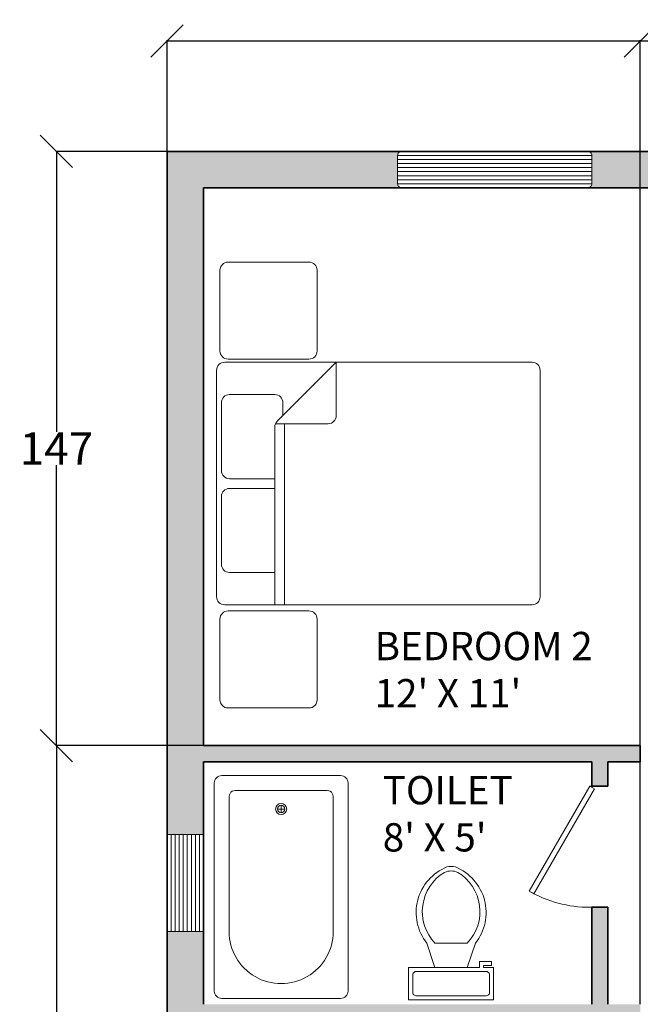
# Model space of a CAD drawing. Units: inches. Extents: x -8 to 447, y -560 to 47.
# Tile 3 of 5: x -8 to 146, y -196 to 47. Entities that reach past the tile are written whole.
import ezdxf

# ---------------------------------------------------------------- set-up
doc = ezdxf.new("R2010")
doc.units = ezdxf.units.IN
doc.header["$MEASUREMENT"] = 0
for name, color, linetype, lineweight in [('A-ANNO-DIMS', 2, 'Continuous', 18), ('A-AREA-IDEN', 7, 'Continuous', 18), ('A-FLOR-FIXT', 8, 'Continuous', 18), ('A-FURN', 8, 'Continuous', 18), ('A-WALL', 7, 'Continuous', 35), ('A-WALL-PATT', 251, 'Continuous', 13), ('DOOR', 40, 'Continuous', 18), ('WINDOW', 151, 'Continuous', 13)]:
    doc.layers.add(name, color=color, linetype=linetype, lineweight=lineweight)
doc.styles.get("Standard").update_dxf_attribs({"font": 'arial.ttf'})
doc.dimstyles.get("Standard").update_dxf_attribs({"dimtxt": 8, "dimasz": 8, "dimexe": 0.18, "dimexo": 0.0625, "dimgap": 0.09, "dimtad": 0, "dimtih": 1, "dimtoh": 1, "dimdec": 0, "dimzin": 0, "dimdsep": 46, "dimlunit": 4, "dimtxsty": 'Standard', "dimblk": 'OBLIQUE', "dimcen": 0.09, "dimadec": 0, "dimazin": 0, "dimtfac": 1, "dimtdec": 0, "dimtofl": 0, "dimtmove": 0, "dimatfit": 3, "dimldrblk": 'OBLIQUE', "dimfxl": 1, "dimtolj": 1, "dimtzin": 0, "dimarcsym": 0})

# ---------------------------------------------------------------- blocks, each defined once
blk = doc.blocks.new('WINDOW')
for p, q in [((0, -1.63), (48, -1.63)), ((0, -2.63), (48, -2.63)), ((0, -3.63), (48, -3.63)), ((0, -4.63), (48, -4.63)), ((0, -5.63), (48, -5.63)), ((0, -6.63), (48, -6.63)), ((0, -7.63), (48, -7.63)), ((0, -8.63), (48, -8.63))]:
    blk.add_line(p, q)
blk.add_lwpolyline([(48, -1.63), (48, -8.63, -0.414214), (47, -9.63), (1, -9.63, -0.414214), (0, -8.63), (0, -1.63, -0.414214), (1, -0.63), (47, -0.63, -0.414214)], format="xyb", close=True)
blk = doc.blocks.new('*U4')
for p, q in [((0, 0), (0, 6)), ((40, 0), (40, 6))]:
    blk.add_line(p, q)
blk.add_lwpolyline([(0, 0), (34.64, -20), (35.52, -18.48), (0.87, 1.52)], close=True)
blk.add_arc((0, 0), 40, 330, 0)
blk = doc.blocks.new('Bath Tub - 26 x 60 in.')
for p, q in [((8, -18), (10, -18)), ((9, -17), (9, -19))]:
    blk.add_line(p, q)
blk.add_lwpolyline([(0, -34), (0, -2, -0.414214), (2, 0), (58, 0, -0.414214), (60, -2), (60, -34, -0.414214), (58, -36), (2, -36, -0.414214)], format="xyb", close=True)
for points in [[(6, -4), (42, -4)], [(4, -30), (4, -6)], [(42, -32), (6, -32)]]:
    blk.add_lwpolyline(points)
for radius in [1.5, 1]:
    blk.add_circle((9, -18), radius)
for centre, radius, start, end in [((5.75, -5.75), 1.77, 81.8699, 188.1301), ((42, -18), 14, 270, 90), ((5.75, -30.25), 1.77, 171.8699, 278.1301)]:
    blk.add_arc(centre, radius, start, end)
blk = doc.blocks.new('Toilet - top')
for p, q in [((9.5, -6), (9.5, -2)), ((-10, -8.5), (-8, -8.5)), ((-10, -9.5), (-10, -8.5)), ((-7, -9.5), (-10, -9.5)), ((-8, -8.5), (-8, -8)), ((-7, -8), (-7, -9.5)), ((-4, -8), (-6, -14)), ((4, -8), (6, -14)), ((4, -14), (-4, -14))]:
    blk.add_line(p, q)
for points in [[(-7, -8), (10.5, -8), (10.5, 0), (-10.5, 0), (-10.5, -8), (-8, -8)], [(-9.5, -2), (-9.5, -6)], [(8.5, -1), (-8.5, -1)], [(-8.5, -7), (8.5, -7)]]:
    blk.add_lwpolyline(points)
for centre, radius, start, end in [((-8.62, -1.88), 0.884, 81.8699, 188.1301), ((8.62, -1.88), 0.884, 351.8699, 98.1301), ((-8.62, -6.12), 0.884, 171.8699, 278.1301), ((8.62, -6.12), 0.884, 261.8699, 8.1301), ((3.52, -21.58), 12.17, 141.4691, 247.9714), ((4.2, -21.82), 11.33, 136.3677, 238.9468), ((-3.52, -21.58), 12.17, 292.0284, 38.5307), ((-4.2, -21.82), 11.33, 301.053, 43.6321), ((0, -27.88), 4, 245.7318, 294.2682), ((0, -29), 4, 254.8605, 285.1395)]:
    blk.add_arc(centre, radius, start, end)
blk = doc.blocks.new('Bed - Queen')
for p, q in [((2, 0), (58, 0)), ((0, -78), (0, -2)), ((10, -1.2), (26.8, -1.2)), ((33.2, -1.2), (50, -1.2)), ((60, -2), (60, -78)), ((8, -14.4), (8, -3.2)), ((28.8, -3.2), (28.8, -14.4)), ((31.2, -14.4), (31.2, -3.2)), ((52, -3.2), (52, -14.4)), ((0, -14.4), (43.97, -14.4)), ((44.8, -14.58), (44.8, -27.6)), ((44.8, -16.8), (0, -16.8)), ((60, -29.6), (45.39, -14.99)), ((50, -16.4), (46.8, -16.4)), ((46.8, -29.6), (60, -29.6)), ((58, -80), (2, -80))]:
    blk.add_line(p, q)
for centre, start, end in [((2, -2), 90, 180), ((58, -2), 0, 90), ((10, -3.2), 90, 180), ((26.8, -3.2), 0, 90), ((33.2, -3.2), 90, 180), ((50, -3.2), 0, 90), ((43.97, -16.4), 45, 90), ((50, -14.4), 270, 0), ((46.8, -27.6), 180, 270), ((2, -78), 180, 270), ((58, -78), 270, 0)]:
    blk.add_arc(centre, 2, start, end)
blk = doc.blocks.new('WIN-24IN-GLAZING')
for p, q in [((0, 9), (24, 9)), ((0, 8), (24, 8)), ((0, 7), (24, 7)), ((0, 6), (24, 6)), ((0, 5), (24, 5)), ((0, 4), (24, 4)), ((0, 3), (24, 3)), ((0, 2), (24, 2)), ((0, 1), (24, 1)), ((24, 0), (0, 0))]:
    blk.add_line(p, q)
blk = doc.blocks.new('NIGHTSTAND-24IN')
blk.add_lwpolyline([(22, 0), (2, 0, -0.414214), (0, 2), (0, 22, -0.414214), (2, 24), (22, 24, -0.414214), (24, 22), (24, 2, -0.414214)], format="xyb", close=True)
blk = doc.blocks.new('_Oblique')
at = {"color": 0, "linetype": 'ByBlock', "lineweight": -2}
blk.add_line((-0.5, -0.5), (0.5, 0.5), dxfattribs=at)
blk = doc.blocks.new('*D51')
at = {"layer": 'A-ANNO-DIMS', "color": 0, "lineweight": -2, "transparency": 16777216}
for p, q in [((28.7, 14.62), (28.7, 42.09)), ((28.7, 41.91), (194.79, 41.91)), ((378.7, 41.91), (212.61, 41.91)), ((378.7, 14.62), (378.7, 42.09))]:
    blk.add_line(p, q, dxfattribs=at)
at = {"layer": 'Defpoints', "color": 0, "transparency": 16777216}
for p in [(378.7, 41.91), (28.7, 14.56), (378.7, 14.56)]:
    blk.add_point(p, dxfattribs=at)
at = {"layer": 'A-ANNO-DIMS', "color": 0, "lineweight": -2, "transparency": 16777216, "xscale": 8, "yscale": 8, "zscale": 8, "rotation": 180}
blk.add_blockref('_Oblique', (28.7, 41.91), dxfattribs=at)
at = {"layer": 'A-ANNO-DIMS', "color": 0, "lineweight": -2, "transparency": 16777216, "xscale": 8, "yscale": 8, "zscale": 8}
blk.add_blockref('_Oblique', (378.7, 41.91), dxfattribs=at)
at = {"layer": 'A-ANNO-DIMS', "color": 0, "transparency": 16777216, "insert": (203.7, 41.91), "char_height": 8, "attachment_point": 5}
blk.add_mtext('\\A1;350', dxfattribs=at)
blk = doc.blocks.new('*D53')
at = {"layer": 'A-ANNO-DIMS', "color": 0, "lineweight": -2, "transparency": 16777216}
for p, q in [((28.64, 14.56), (1.17, 14.56)), ((1.35, 14.56), (1.35, -54.83)), ((1.35, -132.44), (1.35, -63.05)), ((37.64, -132.44), (1.17, -132.44))]:
    blk.add_line(p, q, dxfattribs=at)
at = {"layer": 'Defpoints', "color": 0, "transparency": 16777216}
for p in [(28.7, 14.56), (1.35, -132.44), (37.7, -132.44)]:
    blk.add_point(p, dxfattribs=at)
at = {"layer": 'A-ANNO-DIMS', "color": 0, "lineweight": -2, "transparency": 16777216, "xscale": 8, "yscale": 8, "zscale": 8}
for p, rotation in [((1.35, 14.56), 90), ((1.35, -132.44), 270)]:
    blk.add_blockref('_Oblique', p, dxfattribs=dict(at, rotation=rotation))
at = {"layer": 'A-ANNO-DIMS', "color": 0, "transparency": 16777216, "insert": (1.35, -58.94), "char_height": 8, "attachment_point": 5}
blk.add_mtext('\\A1;147', dxfattribs=at)
blk = doc.blocks.new('*D54')
at = {"layer": 'A-ANNO-DIMS', "color": 0, "lineweight": -2, "transparency": 16777216}
for p, q in [((37.64, -132.44), (1.17, -132.44)), ((1.35, -132.44), (1.35, -230.27)), ((1.35, -336.44), (1.35, -238.61)), ((37.64, -336.44), (1.17, -336.44))]:
    blk.add_line(p, q, dxfattribs=at)
at = {"layer": 'Defpoints', "color": 0, "transparency": 16777216}
for p in [(37.7, -132.44), (1.35, -336.44), (37.7, -336.44)]:
    blk.add_point(p, dxfattribs=at)
at = {"layer": 'A-ANNO-DIMS', "color": 0, "lineweight": -2, "transparency": 16777216, "xscale": 8, "yscale": 8, "zscale": 8}
for p, rotation in [((1.35, -132.44), 90), ((1.35, -336.44), 270)]:
    blk.add_blockref('_Oblique', p, dxfattribs=dict(at, rotation=rotation))
at = {"layer": 'A-ANNO-DIMS', "color": 0, "transparency": 16777216, "insert": (1.35, -234.44), "char_height": 8, "attachment_point": 5}
blk.add_mtext('\\A1;204', dxfattribs=at)
blk = doc.blocks.new('*D68')
at = {"layer": 'A-ANNO-DIMS', "color": 0, "lineweight": -2, "transparency": 16777216}
for p, q in [((145.7, -196.38), (145.7, 42.09)), ((145.7, 41.91), (154.9, 41.91)), ((175.7, 41.91), (166.51, 41.91)), ((175.7, -196.38), (175.7, 42.09))]:
    blk.add_line(p, q, dxfattribs=at)
at = {"layer": 'Defpoints', "color": 0, "transparency": 16777216}
for p in [(175.7, 41.91), (145.7, -196.44), (175.7, -196.44)]:
    blk.add_point(p, dxfattribs=at)
at = {"layer": 'A-ANNO-DIMS', "color": 0, "lineweight": -2, "transparency": 16777216, "xscale": 8, "yscale": 8, "zscale": 8, "rotation": 180}
blk.add_blockref('_Oblique', (145.7, 41.91), dxfattribs=at)
at = {"layer": 'A-ANNO-DIMS', "color": 0, "lineweight": -2, "transparency": 16777216, "xscale": 8, "yscale": 8, "zscale": 8}
blk.add_blockref('_Oblique', (175.7, 41.91), dxfattribs=at)
at = {"layer": 'A-ANNO-DIMS', "color": 0, "transparency": 16777216, "insert": (160.7, 41.91), "char_height": 8, "attachment_point": 5}
blk.add_mtext('\\A1;30', dxfattribs=at)

msp = doc.modelspace()

# ---------------------------------------------------------------- hatches: boundary and pattern name
at = {"layer": 'A-WALL-PATT'}
h = msp.add_hatch(color=256, dxfattribs=at)
h.dxf.hatch_style = 1
h.paths.add_polyline_path([(85.702, 14.56), (28.702, 14.56), (28.702, -154.44), (37.702, -154.44), (37.702, -136.44), (133.702, -136.44), (133.702, -142.44), (137.702, -142.44), (137.702, -136.44), (145.702, -136.44), (145.702, -132.44), (37.702, -132.44), (37.702, 5.56), (85.702, 5.56)])
h = msp.add_hatch(color=256, dxfattribs=at)
h.dxf.hatch_style = 1
h.paths.add_polyline_path([(378.702, 14.56), (333.702, 14.56), (333.702, 5.56), (369.702, 5.56), (369.702, -90.44), (321.702, -90.44), (321.702, -94.44), (369.702, -94.44), (369.702, -154.733), (378.702, -154.733)])
h.paths.add_polyline_path([(285.702, 14.56), (227.702, 14.56), (227.702, 5.56), (245.702, 5.56), (245.702, -90.44), (239.702, -90.44), (239.702, -94.44), (249.702, -94.44), (249.702, -90.44), (249.702, 5.56), (285.702, 5.56)])
h.paths.add_polyline_path([(203.702, 14.56), (133.702, 14.56), (133.702, 5.56), (181.702, 5.56), (181.702, -132.44), (175.702, -132.44), (175.702, -136.44), (185.702, -136.44), (185.702, -94.44), (209.702, -94.44), (209.702, -90.44), (185.702, -90.44), (185.702, 5.56), (203.702, 5.56)])
h = msp.add_hatch(color=256, dxfattribs=at)
h.dxf.hatch_style = 1
h.paths.add_polyline_path([(37.702, -178.44), (28.702, -178.44), (28.702, -238.368), (37.702, -238.368), (37.702, -200.44), (145.702, -200.44), (145.702, -196.44), (137.702, -196.44), (137.702, -172.44), (133.702, -172.44), (133.702, -196.44), (37.702, -196.44)])

# ---------------------------------------------------------------- linework, layer by layer
at = {"layer": 'A-WALL'}
for p, q in [((28.702, 14.56), (378.702, 14.56)), ((28.702, -525.44), (28.702, 14.56)), ((37.702, 5.56), (181.702, 5.56)), ((37.702, -132.44), (37.702, 5.56)), ((145.702, -132.44), (37.702, -132.44)), ((145.702, -132.44), (145.702, -136.44)), ((37.702, -196.44), (37.702, -136.44)), ((133.702, -136.44), (37.702, -136.44)), ((133.702, -142.44), (133.702, -136.44)), ((137.702, -142.44), (137.702, -136.44)), ((145.702, -136.44), (137.702, -136.44)), ((133.702, -142.44), (137.702, -142.44)), ((133.702, -196.44), (133.702, -172.44)), ((133.702, -172.44), (137.702, -172.44)), ((137.702, -196.44), (137.702, -172.44))]:
    msp.add_line(p, q, dxfattribs=at)
at = {"layer": 'WINDOW'}
for p, q in [((28.702, -154.44), (37.702, -154.44)), ((37.702, -178.44), (28.702, -178.44))]:
    msp.add_line(p, q, dxfattribs=at)

# ---------------------------------------------------------------- block references
at = {"layer": 'A-FLOR-FIXT', "xscale": 0.9191238910175982, "yscale": 0.9191238910175982, "zscale": 0.9191238910175982, "rotation": 270}
msp.add_blockref('Bath Tub - 26 x 60 in.', (73.451, -139.848), dxfattribs=at)
at = {"layer": 'A-FLOR-FIXT', "rotation": 180}
msp.add_blockref('Toilet - top', (98.931, -195.321), dxfattribs=at)
at = {"layer": 'A-FURN'}
for name, p, rotation in [('NIGHTSTAND-24IN', (41.786, -12.809), 270), ('Bed - Queen', (40.942, -97.594), 90), ('NIGHTSTAND-24IN', (41.786, -99.127), 270)]:
    msp.add_blockref(name, p, dxfattribs=dict(at, rotation=rotation))
at = {"layer": 'DOOR', "xscale": 0.75, "yscale": 0.75, "zscale": 0.75, "rotation": 270}
msp.add_blockref('*U4', (133.202, -142.44), dxfattribs=at)
at = {"layer": 'WINDOW'}
msp.add_blockref('WINDOW', (85.702, 15.195), dxfattribs=at)
at = {"layer": 'WINDOW', "rotation": 89.99999999999996}
msp.add_blockref('WIN-24IN-GLAZING', (37.702, -178.44), dxfattribs=at)

# ---------------------------------------------------------------- texts
at = {"layer": 'A-AREA-IDEN', "char_height": 7, "attachment_point": 1}
for s, width, insert in [("BEDROOM 2\\P12' X 11'", 136.8374, (80.018, -104.303)), ("TOILET\\P8' X 5' ", 82.35562, (82.032, -139.963))]:
    msp.add_mtext_dynamic_manual_height_columns(s, width=width, gutter_width=1, heights=[0], dxfattribs=dict(at, insert=insert))

# ---------------------------------------------------------------- dimensions: what is measured, and where the dimension line sits
at = {"layer": 'A-ANNO-DIMS'}
for base, p1, p2, picture, middle in [((378.702, 41.91), (28.702, 14.56), (378.702, 14.56), '*D51', (203.702, 41.91)), ((175.702, 41.91), (145.702, -196.44), (175.702, -196.44), '*D68', (160.702, 41.91))]:
    dim = msp.add_linear_dim(base=base, p1=p1, p2=p2, dimstyle='Standard', override={"dimdec": 0, "dimlfac": 1, "dimrnd": 0, "dimzin": 0, "dimdsep": 46, "dimlunit": 2}, dxfattribs=at)
    dim.commit()
    dim.dimension.update_dxf_attribs({"geometry": picture, "text_midpoint": middle})
for base, p1, p2, picture, middle in [((1.352, -132.44), (28.702, 14.56), (37.702, -132.44), '*D53', (1.352, -58.94)), ((1.352, -336.44), (37.702, -132.44), (37.702, -336.44), '*D54', (1.352, -234.44))]:
    dim = msp.add_linear_dim(base=base, p1=p1, p2=p2, angle=90, dimstyle='Standard', override={"dimdec": 0, "dimlfac": 1, "dimrnd": 0, "dimzin": 0, "dimdsep": 46, "dimlunit": 2}, dxfattribs=at)
    dim.commit()
    dim.dimension.update_dxf_attribs({"geometry": picture, "text_midpoint": middle})

doc.saveas('drawing.dxf')
